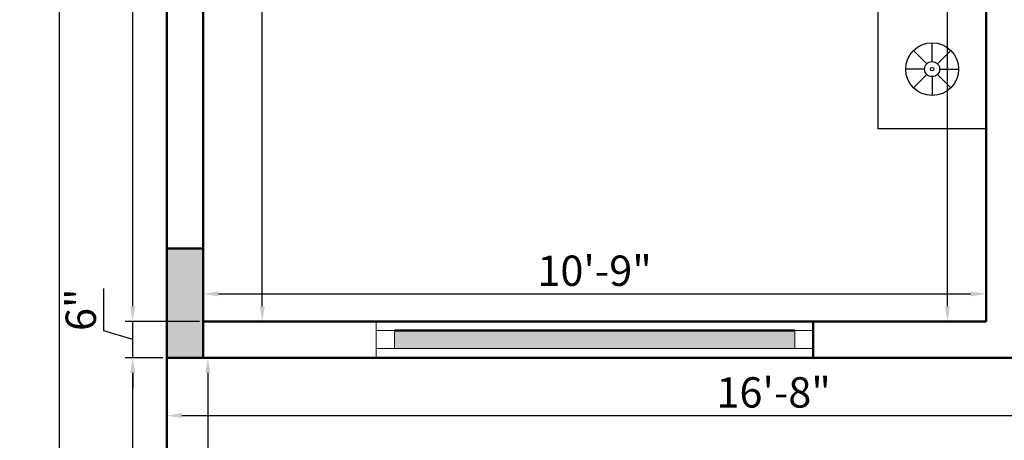
# Model space of a CAD drawing. Units: inches. Extents: x 3064 to 19385, y 846 to 15425.
# Tile 93 of 108: x 7502 to 7664, y 963 to 1032. Entities that reach past the tile are written whole.
import ezdxf

# ---------------------------------------------------------------- set-up
doc = ezdxf.new("R2010")
doc.units = ezdxf.units.IN
for name, color, linetype, lineweight in [('A-ANNO-DIMS', 2, 'Continuous', 18), ('A-COLS', 1, 'Continuous', 35), ('A-FLOR-FIXT', 9, 'Continuous', 18), ('A-GLAZ', 4, 'Continuous', 18), ('A-WALL', 7, 'Continuous', 50)]:
    doc.layers.add(name, color=color, linetype=linetype, lineweight=lineweight)
doc.layers.add('BLOCK', color=6, linetype='Continuous')
doc.styles.get("Standard").update_dxf_attribs({"font": 'arial.ttf'})
doc.dimstyles.new('ISO-25', dxfattribs={"dimtxt": 9, "dimasz": 2.5, "dimexe": 1.25, "dimexo": 0.625, "dimtad": 1, "dimdec": 1, "dimlunit": 3, "dimtxsty": 'Standard', "dimcen": 2.5, "dimadec": 0, "dimazin": 0, "dimtfac": 1, "dimtdec": 1, "dimtmove": 0, "dimatfit": 3, "dimfxl": 1, "dimarcsym": 0})

# ---------------------------------------------------------------- blocks, each defined once
blk = doc.blocks.new('*D316')
at = {"layer": 'A-ANNO-DIMS', "color": 0, "lineweight": -2, "transparency": 16777216}
for p, q in [((7525.62, 976.34), (7519.4, 976.34)), ((7520.65, 906.84), (7520.65, 973.84)), ((7525.62, 904.34), (7519.4, 904.34))]:
    blk.add_line(p, q, dxfattribs=at)
at = {"layer": 'A-ANNO-DIMS', "color": 0, "transparency": 16777216}
for points in [[(7520.23, 973.84), (7521.06, 973.84), (7520.65, 976.34)], [(7520.23, 906.84), (7521.06, 906.84), (7520.65, 904.34)]]:
    blk.add_solid(points, dxfattribs=at)
at = {"layer": 'Defpoints', "color": 0, "transparency": 16777216}
for p in [(7520.65, 976.34), (7526.25, 976.34), (7526.25, 904.34)]:
    blk.add_point(p, dxfattribs=at)
at = {"layer": 'A-ANNO-DIMS', "color": 0, "transparency": 16777216, "insert": (7517.47, 940.34), "char_height": 5, "attachment_point": 5, "rotation": 90}
blk.add_mtext("6'", dxfattribs=at)
blk = doc.blocks.new('*D317')
at = {"layer": 'A-ANNO-DIMS', "color": 0, "lineweight": -2, "transparency": 16777216}
for p, q in [((7515.91, 980.76), (7515.91, 987.79)), ((7520.65, 984.84), (7520.65, 987.34)), ((7531.62, 982.34), (7519.4, 982.34)), ((7520.65, 976.34), (7520.65, 982.34)), ((7520.65, 976.34), (7520.65, 982.34)), ((7520.65, 979.34), (7515.91, 980.76)), ((7525.62, 976.34), (7519.4, 976.34)), ((7520.65, 973.84), (7520.65, 971.34))]:
    blk.add_line(p, q, dxfattribs=at)
at = {"layer": 'A-ANNO-DIMS', "color": 0, "transparency": 16777216}
for points in [[(7520.23, 984.84), (7521.06, 984.84), (7520.65, 982.34)], [(7520.23, 973.84), (7521.06, 973.84), (7520.65, 976.34)]]:
    blk.add_solid(points, dxfattribs=at)
at = {"layer": 'Defpoints', "color": 0, "transparency": 16777216}
for p in [(7520.65, 982.34), (7532.25, 982.34), (7526.25, 976.34)]:
    blk.add_point(p, dxfattribs=at)
at = {"layer": 'A-ANNO-DIMS', "color": 0, "transparency": 16777216, "insert": (7512.73, 984.27), "char_height": 5, "attachment_point": 5, "rotation": 90}
blk.add_mtext('6"', dxfattribs=at)
blk = doc.blocks.new('*D318')
at = {"layer": 'A-ANNO-DIMS', "color": 0, "lineweight": -2, "transparency": 16777216}
for p, q in [((7531.62, 1180.34), (7519.4, 1180.34)), ((7520.65, 984.84), (7520.65, 1177.84)), ((7531.62, 982.34), (7519.4, 982.34))]:
    blk.add_line(p, q, dxfattribs=at)
at = {"layer": 'A-ANNO-DIMS', "color": 0, "transparency": 16777216}
for points in [[(7520.23, 1177.84), (7521.06, 1177.84), (7520.65, 1180.34)], [(7520.23, 984.84), (7521.06, 984.84), (7520.65, 982.34)]]:
    blk.add_solid(points, dxfattribs=at)
at = {"layer": 'Defpoints', "color": 0, "transparency": 16777216}
for p in [(7520.65, 1180.34), (7532.25, 1180.34), (7532.25, 982.34)]:
    blk.add_point(p, dxfattribs=at)
at = {"layer": 'A-ANNO-DIMS', "color": 0, "transparency": 16777216, "insert": (7517.47, 1081.34), "char_height": 5, "attachment_point": 5, "rotation": 90}
blk.add_mtext('16\'-6"', dxfattribs=at)
blk = doc.blocks.new('*D324')
at = {"layer": 'A-ANNO-DIMS', "color": 0, "lineweight": -2, "transparency": 16777216}
for p, q in [((7525.62, 1396.34), (7507.31, 1396.34)), ((7508.56, 906.84), (7508.56, 1393.84)), ((7525.62, 904.34), (7507.31, 904.34))]:
    blk.add_line(p, q, dxfattribs=at)
at = {"layer": 'A-ANNO-DIMS', "color": 0, "transparency": 16777216}
for points in [[(7508.15, 1393.84), (7508.98, 1393.84), (7508.56, 1396.34)], [(7508.15, 906.84), (7508.98, 906.84), (7508.56, 904.34)]]:
    blk.add_solid(points, dxfattribs=at)
at = {"layer": 'Defpoints', "color": 0, "transparency": 16777216}
for p in [(7508.56, 1396.34), (7526.25, 1396.34), (7526.25, 904.34)]:
    blk.add_point(p, dxfattribs=at)
at = {"layer": 'A-ANNO-DIMS', "color": 0, "transparency": 16777216, "insert": (7505.43, 1150.34), "char_height": 5, "attachment_point": 5, "rotation": 90}
blk.add_mtext("41'", dxfattribs=at)
blk = doc.blocks.new('*D265')
at = {"layer": 'A-ANNO-DIMS', "color": 0, "lineweight": -2, "transparency": 16777216}
for p, q in [((7526.25, 975.71), (7526.25, 965.55)), ((7726.25, 975.71), (7726.25, 965.55)), ((7528.75, 966.8), (7723.75, 966.8))]:
    blk.add_line(p, q, dxfattribs=at)
at = {"layer": 'A-ANNO-DIMS', "color": 0, "transparency": 16777216}
for points in [[(7528.75, 967.22), (7528.75, 966.39), (7526.25, 966.8)], [(7723.75, 967.22), (7723.75, 966.39), (7726.25, 966.8)]]:
    blk.add_solid(points, dxfattribs=at)
at = {"layer": 'Defpoints', "color": 0, "transparency": 16777216}
for p in [(7526.25, 976.34), (7726.25, 976.34), (7726.25, 966.8)]:
    blk.add_point(p, dxfattribs=at)
at = {"layer": 'A-ANNO-DIMS', "color": 0, "transparency": 16777216, "insert": (7626.25, 969.98), "char_height": 5, "attachment_point": 5}
blk.add_mtext('16\'-8"', dxfattribs=at)
blk = doc.blocks.new('*D220')
at = {"layer": 'A-ANNO-DIMS', "color": 0, "lineweight": -2, "transparency": 16777216}
for p, q in [((7526.87, 976.34), (7534.27, 976.34)), ((7533.02, 973.84), (7533.02, 906.84)), ((7526.87, 904.34), (7534.27, 904.34))]:
    blk.add_line(p, q, dxfattribs=at)
at = {"layer": 'A-ANNO-DIMS', "color": 0, "transparency": 16777216}
for points in [[(7532.61, 973.84), (7533.44, 973.84), (7533.02, 976.34)], [(7532.61, 906.84), (7533.44, 906.84), (7533.02, 904.34)]]:
    blk.add_solid(points, dxfattribs=at)
at = {"layer": 'Defpoints', "color": 0, "transparency": 16777216}
for p in [(7526.25, 976.34), (7526.25, 904.34), (7533.02, 904.34)]:
    blk.add_point(p, dxfattribs=at)
at = {"layer": 'A-ANNO-DIMS', "color": 0, "transparency": 16777216, "insert": (7529.85, 940.34), "char_height": 5, "attachment_point": 5, "rotation": 90}
blk.add_mtext("6'", dxfattribs=at)
blk = doc.blocks.new('*D262')
at = {"layer": 'A-ANNO-DIMS', "color": 0, "lineweight": -2, "transparency": 16777216}
for p, q in [((7532.25, 982.96), (7532.25, 988.12)), ((7661.25, 982.96), (7661.25, 988.12)), ((7534.75, 986.87), (7658.75, 986.87))]:
    blk.add_line(p, q, dxfattribs=at)
at = {"layer": 'A-ANNO-DIMS', "color": 0, "transparency": 16777216}
for points in [[(7534.75, 987.29), (7534.75, 986.45), (7532.25, 986.87)], [(7658.75, 987.29), (7658.75, 986.45), (7661.25, 986.87)]]:
    blk.add_solid(points, dxfattribs=at)
at = {"layer": 'Defpoints', "color": 0, "transparency": 16777216}
for p in [(7661.25, 986.87), (7532.25, 982.34), (7661.25, 982.34)]:
    blk.add_point(p, dxfattribs=at)
at = {"layer": 'A-ANNO-DIMS', "color": 0, "transparency": 16777216, "insert": (7596.75, 990.05), "char_height": 5, "attachment_point": 5}
blk.add_mtext('10\'-9"', dxfattribs=at)
blk = doc.blocks.new('*D219')
at = {"layer": 'A-ANNO-DIMS', "color": 0, "lineweight": -2, "transparency": 16777216}
for p, q in [((7532.87, 1180.34), (7543.24, 1180.34)), ((7541.99, 984.84), (7541.99, 1177.84)), ((7532.87, 982.34), (7543.24, 982.34))]:
    blk.add_line(p, q, dxfattribs=at)
at = {"layer": 'A-ANNO-DIMS', "color": 0, "transparency": 16777216}
for points in [[(7541.58, 1177.84), (7542.41, 1177.84), (7541.99, 1180.34)], [(7541.58, 984.84), (7542.41, 984.84), (7541.99, 982.34)]]:
    blk.add_solid(points, dxfattribs=at)
at = {"layer": 'Defpoints', "color": 0, "transparency": 16777216}
for p in [(7532.25, 1180.34), (7541.99, 1180.34), (7532.25, 982.34)]:
    blk.add_point(p, dxfattribs=at)
at = {"layer": 'A-ANNO-DIMS', "color": 0, "transparency": 16777216, "insert": (7538.82, 1081.34), "char_height": 5, "attachment_point": 5, "rotation": 90}
blk.add_mtext('16\'-6"', dxfattribs=at)
blk = doc.blocks.new('*D234')
at = {"layer": 'A-ANNO-DIMS', "color": 0, "lineweight": -2, "transparency": 16777216}
for p, q in [((7660.62, 1144.34), (7653.63, 1144.34)), ((7654.88, 984.84), (7654.88, 1141.84)), ((7660.62, 982.34), (7653.63, 982.34))]:
    blk.add_line(p, q, dxfattribs=at)
at = {"layer": 'A-ANNO-DIMS', "color": 0, "transparency": 16777216}
for points in [[(7654.46, 1141.84), (7655.29, 1141.84), (7654.88, 1144.34)], [(7654.46, 984.84), (7655.29, 984.84), (7654.88, 982.34)]]:
    blk.add_solid(points, dxfattribs=at)
at = {"layer": 'Defpoints', "color": 0, "transparency": 16777216}
for p in [(7654.88, 1144.34), (7661.25, 1144.34), (7661.25, 982.34)]:
    blk.add_point(p, dxfattribs=at)
at = {"layer": 'A-ANNO-DIMS', "color": 0, "transparency": 16777216, "insert": (7651.7, 1063.34), "char_height": 5, "attachment_point": 5, "rotation": 90}
blk.add_mtext('13\'-6"', dxfattribs=at)
blk = doc.blocks.new('A$C52E67D0D')
at = {"layer": 'BLOCK'}
for p, q in [((2229.3, 1596.3), (2173.3, 1652.3)), ((2251.5, 1605.5), (2251.5, 1684.7)), ((2273.7, 1596.3), (2329.7, 1652.3)), ((2220.1, 1574.1), (2140.9, 1574.1)), ((2282.9, 1574.1), (2362.1, 1574.1)), ((2229.3, 1551.9), (2173.3, 1495.9)), ((2251.5, 1542.8), (2251.5, 1463.5)), ((2273.7, 1551.9), (2329.7, 1495.9))]:
    blk.add_line(p, q, dxfattribs=at)
blk.add_lwpolyline([(2001, 1348.6), (2001, 1799.6), (2502, 1799.6), (2502, 1348.6)], close=True, dxfattribs=at)
for radius in [110.6, 31.4, 7.46]:
    blk.add_circle((2251.5, 1574.1), radius, dxfattribs=at)
blk = doc.blocks.new('WIN-1900')
blk.add_line((3, 0), (3, 66))
blk.add_lwpolyline([(3, 66), (0, 66), (0, 69), (3, 69)], close=True)
blk = doc.blocks.new('*D432')
at = {"layer": 'A-ANNO-DIMS', "color": 0, "lineweight": -2, "transparency": 16777216}
for p, q in [((7527.75, 1044.71), (7527.75, 1033.74)), ((7530.75, 1044.71), (7530.75, 1033.74)), ((7525.25, 1034.99), (7522.75, 1034.99)), ((7527.75, 1034.99), (7530.75, 1034.99)), ((7533.25, 1034.99), (7591.86, 1034.99))]:
    blk.add_line(p, q, dxfattribs=at)
at = {"layer": 'A-ANNO-DIMS', "color": 0, "transparency": 16777216}
for points in [[(7525.25, 1035.41), (7525.25, 1034.57), (7527.75, 1034.99)], [(7533.25, 1035.41), (7533.25, 1034.57), (7530.75, 1034.99)]]:
    blk.add_solid(points, dxfattribs=at)
at = {"layer": 'Defpoints', "color": 0, "transparency": 16777216}
for p in [(7527.75, 1045.34), (7530.75, 1045.34), (7530.75, 1034.99)]:
    blk.add_point(p, dxfattribs=at)
at = {"layer": 'A-ANNO-DIMS', "color": 0, "transparency": 16777216, "insert": (7563.8, 1040.21), "char_height": 9, "attachment_point": 5}
blk.add_mtext('0\'-3" TYP.', dxfattribs=at)

msp = doc.modelspace()

# ---------------------------------------------------------------- hatches: boundary and pattern name
at = {"layer": 'A-COLS'}
h = msp.add_hatch(color=256, dxfattribs=at)
h.dxf.hatch_style = 1
h.paths.add_polyline_path([(7526.25, 976.34), (7532.25, 976.34), (7532.25, 994.34), (7526.25, 994.34)])
at = {"layer": 'A-GLAZ'}
h = msp.add_hatch(color=256, dxfattribs=at)
h.dxf.hatch_style = 1
h.paths.add_polyline_path([(7563.75, 980.84), (7563.75, 977.84), (7629.75, 977.84), (7629.75, 980.84)])

# ---------------------------------------------------------------- linework, layer by layer
msp.add_line((7560.75, 976.34), (7560.75, 982.34), dxfattribs=at)
msp.add_lwpolyline([(7560.75, 977.84), (7560.75, 980.84), (7563.75, 980.84), (7563.75, 977.84)], close=True, dxfattribs=at)
at = {"layer": 'A-WALL'}
for p, q in [((7526.25, 1396.34), (7526.25, 976.34)), ((7532.25, 1180.34), (7532.25, 982.34)), ((7661.25, 1144.34), (7661.25, 982.34)), ((7661.25, 982.34), (7532.25, 982.34)), ((7632.75, 976.34), (7632.75, 982.34)), ((7563.75, 980.84), (7629.75, 980.84)), ((7868.25, 976.34), (7526.25, 976.34)), ((7532.25, 976.34), (7526.25, 976.34)), ((7526.25, 976.34), (7526.25, 904.34))]:
    msp.add_line(p, q, dxfattribs=at)
msp.add_lwpolyline([(7532.25, 976.34), (7532.25, 994.34), (7526.25, 994.34), (7526.25, 976.34)], close=True, dxfattribs=at)

# ---------------------------------------------------------------- block references
at = {"layer": 'A-FLOR-FIXT', "xscale": 0.039370099999992, "yscale": 0.039370099999992, "zscale": 0.039370099999992, "rotation": 270}
msp.add_blockref('A$C52E67D0D', (7590.38, 1112.59), dxfattribs=at)
at = {"layer": 'A-GLAZ', "rotation": 269.9999999999995}
msp.add_blockref('WIN-1900', (7563.75, 980.84), dxfattribs=at)

# ---------------------------------------------------------------- dimensions: what is measured, and where the dimension line sits
at = {"layer": 'A-ANNO-DIMS'}
for base, p1, p2, override, picture, middle in [((7508.56, 1396.34), (7526.25, 904.34), (7526.25, 1396.34), {"dimtxt": 5, "dimclrd": 0, "dimclre": 0, "dimclrt": 0}, '*D324', (7505.43, 1150.34)), ((7520.65, 1180.34), (7532.25, 982.34), (7532.25, 1180.34), {"dimtxt": 5, "dimclrd": 0, "dimclre": 0, "dimclrt": 0, "dimtmove": 1}, '*D318', (7517.47, 1081.34)), ((7541.99, 1180.34), (7532.25, 982.34), (7532.25, 1180.34), {"dimtxt": 5, "dimclrd": 0, "dimclre": 0, "dimclrt": 0}, '*D219', (7538.82, 1081.34)), ((7654.88, 1144.34), (7661.25, 982.34), (7661.25, 1144.34), {"dimtxt": 5, "dimclrd": 0, "dimclre": 0, "dimclrt": 0}, '*D234', (7651.7, 1063.34)), ((7520.65, 982.34), (7526.25, 976.34), (7532.25, 982.34), {"dimtxt": 5, "dimclrd": 0, "dimclre": 0, "dimclrt": 0, "dimtmove": 1}, '*D317', (7512.73, 981.39)), ((7520.65, 976.34), (7526.25, 904.34), (7526.25, 976.34), {"dimtxt": 5, "dimclrd": 0, "dimclre": 0, "dimclrt": 0}, '*D316', (7517.47, 940.34)), ((7533.02, 904.34), (7526.25, 976.34), (7526.25, 904.34), {"dimtxt": 5, "dimclrd": 0, "dimclre": 0, "dimclrt": 0}, '*D220', (7529.85, 940.34))]:
    dim = msp.add_linear_dim(base=base, p1=p1, p2=p2, angle=90, dimstyle='ISO-25', override=override, dxfattribs=at)
    dim.commit()
    dim.dimension.update_dxf_attribs({"geometry": picture, "text_midpoint": middle})
dim = msp.add_linear_dim(base=(7530.75, 1034.99), p1=(7527.75, 1045.34), p2=(7530.75, 1045.34), text='<> TYP.', dimstyle='ISO-25', override={"dimdec": 1, "dimrnd": 0, "dimzin": 1, "dimlunit": 4, "dimfrac": 2}, dxfattribs=at)
dim.commit()
dim.dimension.update_dxf_attribs({"geometry": '*D432', "text_midpoint": (7563.8, 1040.21)})
for base, p1, p2, picture, middle in [((7661.25, 986.87), (7532.25, 982.34), (7661.25, 982.34), '*D262', (7596.75, 990.05)), ((7726.25, 966.8), (7526.25, 976.34), (7726.25, 976.34), '*D265', (7626.25, 969.98))]:
    dim = msp.add_linear_dim(base=base, p1=p1, p2=p2, dimstyle='ISO-25', override={"dimtxt": 5, "dimclrd": 0, "dimclre": 0, "dimclrt": 0}, dxfattribs=at)
    dim.commit()
    dim.dimension.update_dxf_attribs({"geometry": picture, "text_midpoint": middle})

doc.saveas('drawing.dxf')
